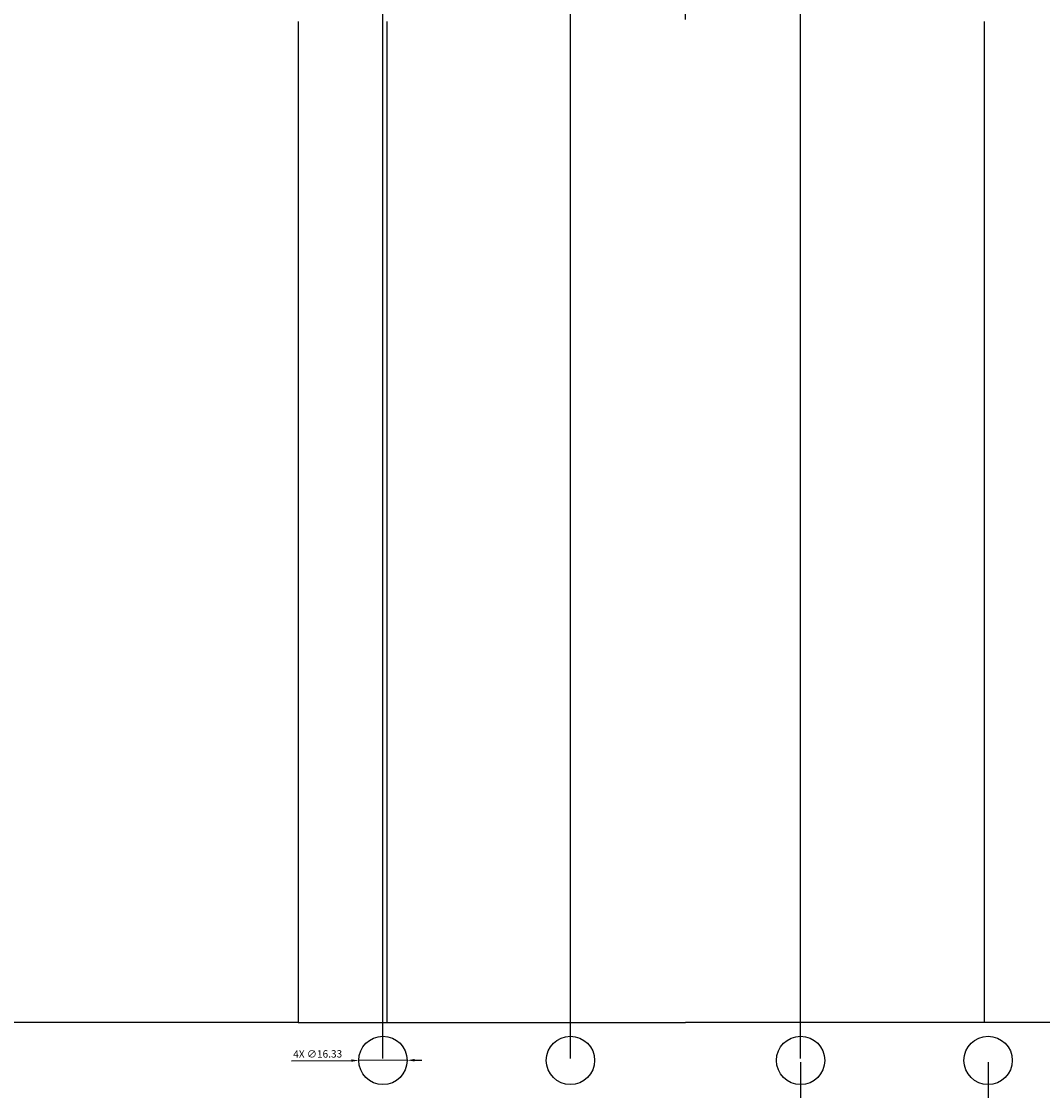
# Model space of a CAD drawing. Units: millimetres. Extents: x 2332 to 5836, y -853 to 2199.
# Tile 10 of 16: x 3986 to 4331, y 1007 to 1368. Entities that reach past the tile are written whole.
import ezdxf

# ---------------------------------------------------------------- set-up
doc = ezdxf.new("R2010")
doc.units = ezdxf.units.MM
doc.layers.get('0').update_dxf_attribs({"color": 8})
doc.layers.add('A-ANNO-DIMS', color=2, linetype='Continuous', lineweight=18)
doc.layers.add('A-EQPM', color=7, linetype='Continuous', lineweight=25)
doc.styles.get("Standard").update_dxf_attribs({"font": 'arial.ttf'})
doc.dimstyles.new('ISO-25', dxfattribs={"dimtxt": 2.5, "dimasz": 2.5, "dimexe": 1.25, "dimexo": 0.625, "dimtad": 1, "dimtxsty": 'Standard', "dimcen": 2.5, "dimadec": 0, "dimazin": 0, "dimtfac": 1, "dimtmove": 0, "dimatfit": 3, "dimfxl": 1, "dimarcsym": 0})

# ---------------------------------------------------------------- blocks, each defined once
blk = doc.blocks.new('HOOD-CONTROL-BUTTON')
blk.add_circle((8.16, 8.16), 8.16)
blk = doc.blocks.new('*D23')
at = {"layer": 'A-ANNO-DIMS', "color": 0, "lineweight": -2, "transparency": 16777216}
for p, q in [((3646.47, 1030.43), (3646.47, 2168.7)), ((3648.97, 2167.45), (4771.11, 2167.45)), ((4773.61, 1030.43), (4773.61, 2168.7))]:
    blk.add_line(p, q, dxfattribs=at)
at = {"layer": 'A-ANNO-DIMS', "color": 0, "transparency": 16777216}
for points in [[(3648.97, 2167.87), (3648.97, 2167.04), (3646.47, 2167.45)], [(4771.11, 2167.87), (4771.11, 2167.04), (4773.61, 2167.45)]]:
    blk.add_solid(points, dxfattribs=at)
at = {"layer": 'Defpoints', "color": 0, "transparency": 16777216}
for p in [(4773.61, 2167.45), (3646.47, 1029.8), (4773.61, 1029.8)]:
    blk.add_point(p, dxfattribs=at)
at = {"layer": 'A-ANNO-DIMS', "color": 0, "transparency": 16777216, "insert": (4210.04, 2169.33), "char_height": 2.5, "attachment_point": 5}
blk.add_mtext('1127.1', dxfattribs=at)
blk = doc.blocks.new('*D30')
at = {"layer": 'A-ANNO-DIMS', "color": 0, "lineweight": -2, "transparency": 16777216}
for p, q in [((3635.04, 1368.43), (3635.04, 2168.7)), ((3637.54, 2167.45), (4207.54, 2167.45)), ((4210.04, 1368.43), (4210.04, 2168.7))]:
    blk.add_line(p, q, dxfattribs=at)
at = {"layer": 'A-ANNO-DIMS', "color": 0, "transparency": 16777216}
for points in [[(3637.54, 2167.87), (3637.54, 2167.04), (3635.04, 2167.45)], [(4207.54, 2167.87), (4207.54, 2167.04), (4210.04, 2167.45)]]:
    blk.add_solid(points, dxfattribs=at)
at = {"layer": 'Defpoints', "color": 0, "transparency": 16777216}
for p in [(4210.04, 2167.45), (3635.04, 1367.8), (4210.04, 1367.8)]:
    blk.add_point(p, dxfattribs=at)
at = {"layer": 'A-ANNO-DIMS', "color": 0, "transparency": 16777216, "insert": (3922.54, 2169.35), "char_height": 2.5, "attachment_point": 5}
blk.add_mtext('575', dxfattribs=at)
blk = doc.blocks.new('*D31')
at = {"layer": 'A-ANNO-DIMS', "color": 0, "lineweight": -2, "transparency": 16777216}
for p, q in [((4171.16, 1017.67), (4171.16, 2168.7)), ((4173.66, 2167.45), (4246.42, 2167.45)), ((4248.92, 1017.67), (4248.92, 2168.7))]:
    blk.add_line(p, q, dxfattribs=at)
at = {"layer": 'A-ANNO-DIMS', "color": 0, "transparency": 16777216}
for points in [[(4173.66, 2167.87), (4173.66, 2167.04), (4171.16, 2167.45)], [(4246.42, 2167.87), (4246.42, 2167.04), (4248.92, 2167.45)]]:
    blk.add_solid(points, dxfattribs=at)
at = {"layer": 'Defpoints', "color": 0, "transparency": 16777216}
for p in [(4248.92, 2167.45), (4171.16, 1017.04), (4248.92, 1017.04)]:
    blk.add_point(p, dxfattribs=at)
at = {"layer": 'A-ANNO-DIMS', "color": 0, "transparency": 16777216, "insert": (4210.04, 2169.35), "char_height": 2.5, "attachment_point": 5}
blk.add_mtext('77.75', dxfattribs=at)
blk = doc.blocks.new('*D32')
at = {"layer": 'A-ANNO-DIMS', "color": 0, "lineweight": -2, "transparency": 16777216}
for p, q in [((4107.84, 1017.67), (4107.84, 2168.7)), ((4110.34, 2167.45), (4168.66, 2167.45)), ((4171.16, 1017.67), (4171.16, 2168.7))]:
    blk.add_line(p, q, dxfattribs=at)
at = {"layer": 'A-ANNO-DIMS', "color": 0, "transparency": 16777216}
for points in [[(4110.34, 2167.87), (4110.34, 2167.04), (4107.84, 2167.45)], [(4168.66, 2167.87), (4168.66, 2167.04), (4171.16, 2167.45)]]:
    blk.add_solid(points, dxfattribs=at)
at = {"layer": 'Defpoints', "color": 0, "transparency": 16777216}
for p in [(4171.16, 2167.45), (4107.84, 1017.04), (4171.16, 1017.04)]:
    blk.add_point(p, dxfattribs=at)
at = {"layer": 'A-ANNO-DIMS', "color": 0, "transparency": 16777216, "insert": (4139.5, 2169.36), "char_height": 2.5, "attachment_point": 5}
blk.add_mtext('63.33', dxfattribs=at)
blk = doc.blocks.new('*D33')
at = {"layer": 'A-ANNO-DIMS', "color": 0, "lineweight": -2, "transparency": 16777216}
for p, q in [((4248.92, 1016.42), (4248.92, -853.1)), ((4312.24, 1016.42), (4312.24, -853.1)), ((4251.42, -851.85), (4309.74, -851.85))]:
    blk.add_line(p, q, dxfattribs=at)
at = {"layer": 'A-ANNO-DIMS', "color": 0, "transparency": 16777216}
for points in [[(4251.42, -851.43), (4251.42, -852.26), (4248.92, -851.85)], [(4309.74, -851.43), (4309.74, -852.26), (4312.24, -851.85)]]:
    blk.add_solid(points, dxfattribs=at)
at = {"layer": 'Defpoints', "color": 0, "transparency": 16777216}
for p in [(4248.92, 1017.04), (4312.24, 1017.04), (4312.24, -851.85)]:
    blk.add_point(p, dxfattribs=at)
at = {"layer": 'A-ANNO-DIMS', "color": 0, "transparency": 16777216, "insert": (4280.58, -849.94), "char_height": 2.5, "attachment_point": 5}
blk.add_mtext('63.33', dxfattribs=at)
blk = doc.blocks.new('*D34')
at = {"layer": 'A-ANNO-DIMS', "color": 0, "lineweight": -2, "transparency": 16777216}
for p, q in [((4076.93, 1016.87), (4097.17, 1016.98)), ((4116, 1017.09), (4099.67, 1017)), ((4118.5, 1017.11), (4121, 1017.12))]:
    blk.add_line(p, q, dxfattribs=at)
at = {"layer": 'A-ANNO-DIMS', "color": 0, "transparency": 16777216}
for points in [[(4097.17, 1017.4), (4097.17, 1016.57), (4099.67, 1017)], [(4118.5, 1017.52), (4118.5, 1016.69), (4116, 1017.09)]]:
    blk.add_solid(points, dxfattribs=at)
at = {"layer": 'Defpoints', "color": 0, "transparency": 16777216}
for p in [(4099.67, 1017), (4116, 1017.09)]:
    blk.add_point(p, dxfattribs=at)
at = {"layer": 'A-ANNO-DIMS', "color": 0, "transparency": 16777216, "insert": (4085.79, 1018.89), "char_height": 2.5, "attachment_point": 5, "rotation": 0.3276}
blk.add_mtext('4X ∅16.33', dxfattribs=at)

msp = doc.modelspace()

# ---------------------------------------------------------------- linework, layer by layer
at = {"layer": 'A-EQPM'}
for p, q in [((4079.186, 1367.803), (4079.186, 1029.801)), ((4109.186, 1367.803), (4109.186, 1029.801)), ((4310.894, 1367.803), (4310.894, 1029.801)), ((4079.186, 1029.801), (3646.468, 1029.801)), ((4079.186, 1029.801), (4210.04, 1029.801)), ((4340.894, 1029.801), (4210.04, 1029.801))]:
    msp.add_line(p, q, dxfattribs=at)

# ---------------------------------------------------------------- block references
for p in [(4099.672, 1008.88), (4162.998, 1008.88), (4240.752, 1008.88), (4304.078, 1008.88)]:
    msp.add_blockref('HOOD-CONTROL-BUTTON', p, dxfattribs=at)

# ---------------------------------------------------------------- dimensions: what is measured, and where the dimension line sits
at = {"layer": 'A-ANNO-DIMS'}
for base, p1, p2, override, picture, middle in [((4210.04, 2167.453), (3635.04, 1367.803), (4210.04, 1367.803), {"dimdec": 0, "dimlfac": 1, "dimrnd": 0, "dimzin": 0, "dimdsep": 46, "dimlunit": 2}, '*D30', (3922.54, 2169.35)), ((4773.612, 2167.453), (3646.468, 1029.801), (4773.612, 1029.801), {"dimdec": 1, "dimlfac": 1, "dimrnd": 0, "dimzin": 0, "dimdsep": 46, "dimlunit": 2}, '*D23', (4210.04, 2169.334)), ((4171.163, 2167.453), (4107.837, 1017.045), (4171.163, 1017.045), {"dimdec": 2, "dimlfac": 1, "dimrnd": 0, "dimzin": 0, "dimdsep": 46, "dimlunit": 2}, '*D32', (4139.5, 2169.356)), ((4248.917, 2167.453), (4171.163, 1017.045), (4248.917, 1017.045), {"dimdec": 2, "dimlfac": 1, "dimrnd": 0, "dimzin": 0, "dimdsep": 46, "dimlunit": 2}, '*D31', (4210.04, 2169.35)), ((4312.243, -851.847), (4248.917, 1017.045), (4312.243, 1017.045), {"dimdec": 2, "dimlfac": 1, "dimrnd": 0, "dimzin": 0, "dimdsep": 46, "dimlunit": 2}, '*D33', (4280.58, -849.944))]:
    dim = msp.add_linear_dim(base=base, p1=p1, p2=p2, dimstyle='ISO-25', override=override, dxfattribs=at)
    dim.commit()
    dim.dimension.update_dxf_attribs({"geometry": picture, "text_midpoint": middle})
dim = msp.add_diameter_dim_2p(p1=(4116.001, 1017.091), p2=(4099.672, 1016.998), text='4X <>', dimstyle='ISO-25', override={"dimdec": 2, "dimlfac": 1, "dimrnd": 0, "dimzin": 0, "dimdsep": 46, "dimlunit": 2}, dxfattribs=at)
dim.commit()
dim.dimension.update_dxf_attribs({"geometry": '*D34', "text_midpoint": (4085.8, 1016.919)})

doc.saveas('drawing.dxf')
